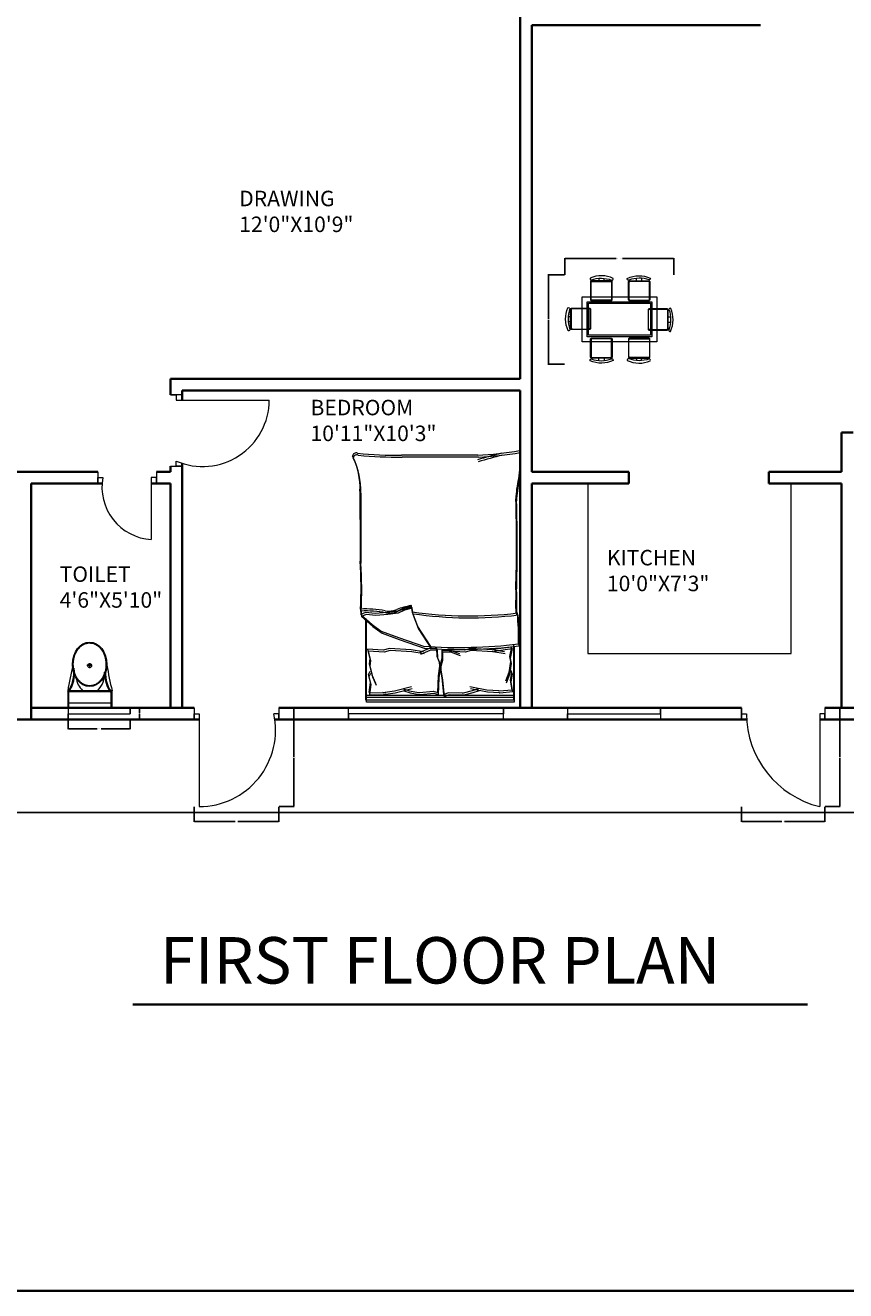
# Model space of a CAD drawing. Units: inches. Extents: x 1520 to 3401, y 1570 to 3432.
# Tile 2 of 15: x 1829 to 2147, y 1570 to 2061. Entities that reach past the tile are written whole.
import ezdxf

# ---------------------------------------------------------------- set-up
doc = ezdxf.new("R2010")
doc.units = ezdxf.units.IN
for name, color, linetype, lineweight in [('A-ANNO-DIMS', 2, 'Continuous', 18), ('A-ANNO-TITL', 7, 'Continuous', 35), ('A-ANNO-TTLB', 7, 'Continuous', 35), ('A-AREA-IDEN', 7, 'Continuous', 18), ('A-DOOR', 3, 'Continuous', 18), ('A-FLOR-CASE', 8, 'Continuous', 18), ('A-FLOR-EDGE', 7, 'Continuous', 25), ('A-FLOR-FIXT', 9, 'Continuous', 18), ('A-FURN', 8, 'Continuous', 13), ('A-GLAZ', 4, 'Continuous', 18), ('A-WALL', 7, 'Continuous', 35)]:
    doc.layers.add(name, color=color, linetype=linetype, lineweight=lineweight)
doc.styles.get("Standard").update_dxf_attribs({"font": 'arial.ttf'})
doc.dimstyles.get("Standard").update_dxf_attribs({"dimtxt": 0.18, "dimasz": 0.18, "dimexe": 0.18, "dimexo": 0.0625, "dimgap": 0.09, "dimtad": 0, "dimtih": 1, "dimtoh": 1, "dimdec": 4, "dimzin": 0, "dimdsep": 46, "dimtxsty": 'Standard', "dimcen": 0.09, "dimadec": 0, "dimazin": 0, "dimtfac": 1, "dimtdec": 4, "dimtofl": 0, "dimtmove": 0, "dimatfit": 3, "dimfxl": 1, "dimtolj": 1, "dimtzin": 0, "dimarcsym": 0})

# ---------------------------------------------------------------- blocks, each defined once
blk = doc.blocks.new('A$C31115884')
for p, q in [((283, 498), (223, 498)), ((258, 466), (258, 523)), ((0, 200), (0, 0)), ((520, 200), (0, 200)), ((10, 190), (10, 10)), ((510, 190), (10, 190)), ((510, 10), (510, 190)), ((520, 0), (520, 200)), ((510, 54), (0, 54)), ((10, 10), (510, 10)), ((0, 0), (520, 0))]:
    blk.add_line(p, q)
blk.add_circle((256, 496), 23.6)
for centre, radius, start, end in [((2778, -205), 2807, 165.4549, 171.7133), ((-295, 403), 365, 324.2091, 9.3499), ((-295, 403), 375, 324.2091, 9.3499), ((806, 403), 365, 170.6501, 215.7909), ((3237, 905), 2807, 188.2867, 194.5451), ((384, 406), 293, 190.2774, 224.1564), ((139, 406), 293, 315.8436, 2.6563), ((806, 403), 375, 179.2036, 215.7909)]:
    blk.add_arc(centre, radius, start, end)
blk.add_ellipse((256, 510), major_axis=(0, -261), ratio=0.772727)
blk.add_open_spline([(256, 259), (263, 259), (270, 260), (288, 262), (299, 265), (320, 273), (330, 278), (350, 291), (360, 299), (378, 316), (386, 326), (402, 347), (409, 358), (421, 383), (427, 395), (436, 422), (440, 436), (445, 465), (447, 480), (448, 509), (448, 524), (445, 553), (443, 568), (436, 596), (432, 610), (422, 636), (416, 649), (402, 672), (395, 683), (379, 703), (370, 712), (351, 728), (341, 735), (321, 746), (310, 751), (289, 757), (278, 759), (256, 761), (245, 761), (223, 757), (212, 754), (191, 746), (181, 741), (161, 728), (151, 720), (133, 703), (125, 693), (110, 672), (103, 660), (90, 636), (85, 623), (76, 596), (72, 582), (67, 553), (66, 538), (64, 509), (65, 494), (68, 465), (70, 450), (77, 422), (81, 408), (91, 382), (97, 370), (111, 346), (118, 335), (135, 316), (144, 307), (162, 291), (172, 284), (193, 273), (203, 269), (225, 262), (236, 260), (250, 259), (253, 259), (256, 259)], degree=3, knots=[0, 0, 0, 0, 0.110105, 0.110105, 0.285049, 0.285049, 0.459994, 0.459994, 0.634938, 0.634938, 0.809882, 0.809882, 0.984827, 0.984827, 1.159771, 1.159771, 1.334715, 1.334715, 1.50966, 1.50966, 1.684604, 1.684604, 1.859549, 1.859549, 2.034493, 2.034493, 2.209437, 2.209437, 2.384382, 2.384382, 2.559326, 2.559326, 2.73427, 2.73427, 2.909215, 2.909215, 3.084159, 3.084159, 3.259103, 3.259103, 3.434048, 3.434048, 3.608992, 3.608992, 3.783936, 3.783936, 3.958881, 3.958881, 4.133825, 4.133825, 4.30877, 4.30877, 4.483714, 4.483714, 4.658658, 4.658658, 4.833603, 4.833603, 5.008547, 5.008547, 5.183491, 5.183491, 5.358436, 5.358436, 5.53338, 5.53338, 5.708324, 5.708324, 5.883269, 5.883269, 6.058213, 6.058213, 6.233158, 6.233158, 6.283185, 6.283185, 6.283185, 6.283185])
blk = doc.blocks.new('DOOR-SWING-24-12')
for p, q in [((0, 26.25), (0, 21.75)), ((22.75, 26.25), (22.75, 21.75)), ((0, 21.75), (0, 24)), ((0, 24), (2, 24)), ((22.75, 24), (20.75, 24)), ((20.75, 24), (20.75, 0)), ((22.75, 21.75), (22.75, 24))]:
    blk.add_line(p, q)
blk.add_arc((21.91, 20.23), 20.26, 169.2703, 266.7379)
blk = doc.blocks.new('DOOR-SWING-36-13')
for p, q in [((4.5, 27.75), (0, 27.75)), ((0, 27.75), (2.25, 27.75)), ((2.25, 27.75), (2.25, 25.75)), ((2.25, 25.75), (38.25, 25.75)), ((0, 0.11), (4.5, 0.11)), ((2.25, 0.11), (2.25, 2.11)), ((4.5, 0.11), (2.25, 0.11))]:
    blk.add_line(p, q)
blk.add_arc((12.49, 25.75), 25.76, 246.5862, 0)
blk = doc.blocks.new('DOOR-SWING-36-28')
for p, q in [((0, 33.75), (0, 38.25)), ((0, 38.25), (0, 33.75)), ((0, 33.75), (0, 36)), ((0, 36), (2, 36)), ((32.37, 36), (30.37, 36)), ((30.37, 36), (30.37, 0)), ((32.37, 38.25), (32.37, 33.75)), ((32.37, 33.75), (32.37, 36))]:
    blk.add_line(p, q)
blk.add_arc((39.03, 36), 37.03, 180, 256.471)
blk = doc.blocks.new('DOOR-SWING-36-29')
for p, q in [((0, 38.25), (0, 34.72)), ((0, 33.75), (0, 36)), ((0, 36), (2, 36)), ((0, 34.72), (0, 33.75)), ((2, 36), (2, 0)), ((32.89, 36), (30.89, 36)), ((32.89, 38.25), (32.89, 33.75)), ((32.89, 33.75), (32.89, 36))]:
    blk.add_line(p, q)
blk.add_arc((2, 29.59), 29.59, 270, 12.5041)
blk = doc.blocks.new('WIN-PLAN-60-02')
for p, q in [((4.5, 60), (0, 60)), ((0, 60), (2.25, 60)), ((2.25, 60), (2.25, 0)), ((4.5, 0), (0, 0)), ((2.25, 0), (4.5, 0))]:
    blk.add_line(p, q)
blk = doc.blocks.new('WIN-PLAN-36-04')
for p, q in [((0, 4.5), (0, 0)), ((0, 0), (0, 2.25)), ((0, 2.25), (36, 2.25)), ((36, 2.25), (36, 4.5)), ((36, 4.5), (36, 0))]:
    blk.add_line(p, q)
blk = doc.blocks.new('WIN-PLAN-24-06')
for p, q in [((0, 4.5), (0, 0)), ((0, 0), (0, 2.25)), ((0, 2.25), (24, 2.25)), ((24, 2.25), (24, 4.5)), ((24, 4.5), (24, 2.25))]:
    blk.add_line(p, q)
blk = doc.blocks.new('KITCHEN-COUNTER-02')
for p, q in [((0, 65.95), (0, 0)), ((78.77, 0), (78.77, 65.95)), ((0, 0), (78.77, 0))]:
    blk.add_line(p, q)
blk = doc.blocks.new('DINING-SET-6-SEAT')
for points in [[(9.94, 32.23, -0.175809), (17.84, 32.17, 0.578392), (18.44, 32.83, 0.214524), (9.52, 32.95, 0.552014), (9.94, 32.23, -0.065079)], [(17.51, 31.92), (10.17, 31.92, 0.414214), (9.66, 31.4), (9.66, 24.66, 0.414214), (10.17, 24.14), (17.51, 24.14, 0.414214), (18.02, 24.66), (18.02, 31.4, 0.414214), (17.51, 31.92)], [(14.93, 31.92), (14.93, 32.84, -0.064759)], [(24.5, 32.17, -0.578392), (23.9, 32.83, -0.214524), (32.82, 32.95, -0.552014), (32.4, 32.23, 0.175809), (24.5, 32.17)], [(32.17, 31.92, -0.414214), (32.68, 31.4), (32.68, 24.66, -0.414214), (32.17, 24.14), (24.83, 24.14, -0.414214), (24.32, 24.66), (24.32, 31.4, -0.414214), (24.83, 31.92), (32.17, 31.92)], [(27.41, 31.92), (27.41, 32.84, 0.064759)], [(1.67, 13.15, -0.578392), (1.02, 12.55, -0.214524), (0.9, 21.47, -0.552014), (1.61, 21.05, 0.175809), (1.67, 13.15)], [(1.93, 20.82, -0.414214), (2.45, 21.33), (9.19, 21.33, -0.414214), (9.7, 20.82), (9.7, 13.49, -0.414214), (9.19, 12.97), (2.45, 12.97, -0.414214), (1.93, 13.49), (1.93, 20.82)], [(39.71, 20.57, 0.414214), (39.19, 21.08), (32.45, 21.08, 0.414214), (31.94, 20.57), (31.94, 13.23, 0.414214), (32.45, 12.72), (39.19, 12.72, 0.414214), (39.71, 13.23), (39.71, 20.57)], [(40.02, 20.8, -0.175809), (39.96, 12.9, 0.578392), (40.62, 12.3, 0.214524), (40.74, 21.22, 0.552014), (40.02, 20.8, -0.065079)], [(1.93, 16.06), (1, 16.06, 0.064759)], [(39.71, 15.81), (40.63, 15.81, -0.064759)], [(17.51, 1.93), (10.17, 1.93, -0.414214), (9.66, 2.45), (9.66, 9.19, -0.414214), (10.17, 9.7), (17.51, 9.7, -0.414214), (18.02, 9.19), (18.02, 2.45, -0.414214), (17.51, 1.93)], [(32.17, 1.93, 0.414214), (32.68, 2.45), (32.68, 9.19, 0.414214), (32.17, 9.7), (24.83, 9.7, 0.414214), (24.32, 9.19), (24.32, 2.45, 0.414214), (24.83, 1.93), (32.17, 1.93)], [(17.84, 1.67, -0.578392), (18.44, 1.02, -0.214524), (9.52, 0.9, -0.552014), (9.94, 1.61, 0.175809), (17.84, 1.67)], [(14.93, 1.93), (14.93, 1, 0.064759)], [(32.4, 1.61, -0.175809), (24.5, 1.67, 0.578392), (23.9, 1.02, 0.214524), (32.82, 0.9, 0.552014), (32.4, 1.61, -0.065079)], [(27.41, 1.93), (27.41, 1, -0.064759)]]:
    blk.add_lwpolyline(points, format="xyb")
for points in [[(10.18, 31.68), (17.28, 31.68, -0.414214), (17.79, 31.17), (17.79, 24.89, -0.414214), (17.28, 24.37), (10.18, 24.37, -0.512069), (9.89, 24.89), (9.89, 31.17, -0.512069)], [(32.16, 31.68), (25.06, 31.68, 0.414214), (24.55, 31.17), (24.55, 24.89, 0.414214), (25.06, 24.37), (32.16, 24.37, 0.512069), (32.45, 24.89), (32.45, 31.17, 0.512069)], [(2.16, 20.82), (2.16, 13.72, 0.414214), (2.68, 13.2), (8.96, 13.2, 0.414214), (9.47, 13.72), (9.47, 20.82, 0.512069), (8.96, 21.1), (2.68, 21.1, 0.512069)], [(39.48, 20.57), (39.48, 13.47, -0.414214), (38.96, 12.95), (32.68, 12.95, -0.414214), (32.17, 13.47), (32.17, 20.57, -0.512069), (32.68, 20.85), (38.96, 20.85, -0.512069)], [(10.18, 2.16), (17.28, 2.16, 0.414214), (17.79, 2.68), (17.79, 8.96, 0.414214), (17.28, 9.47), (10.18, 9.47, 0.512069), (9.89, 8.96), (9.89, 2.68, 0.512069)], [(32.16, 2.16), (25.06, 2.16, -0.414214), (24.55, 2.68), (24.55, 8.96, -0.414214), (25.06, 9.47), (32.16, 9.47, -0.512069), (32.45, 8.96), (32.45, 2.68, -0.512069)]]:
    blk.add_lwpolyline(points, format="xyb", close=True)
for points in [[(12.88, 32.86), (12.88, 31.92)], [(29.46, 32.86), (29.46, 31.92)], [(0.99, 18.12), (1.93, 18.12)], [(40.65, 17.86), (39.71, 17.86)], [(12.88, 0.99), (12.88, 1.93)], [(29.46, 0.99), (29.46, 1.93)]]:
    blk.add_lwpolyline(points)
for points in [[(6.35, 25.72), (35.36, 25.72), (35.36, 8.31), (6.35, 8.31)], [(8.29, 23.79), (33.43, 23.79), (33.43, 10.25), (8.29, 10.25)], [(8.87, 23.21), (32.85, 23.21), (32.85, 10.83), (8.87, 10.83)]]:
    blk.add_lwpolyline(points, close=True)
blk = doc.blocks.new('*D135')
at = {"layer": 'A-ANNO-DIMS', "color": 0, "lineweight": -2, "transparency": 16777216}
for p, q in [((2139.24, 1796.18), (2145.09, 1796.18)), ((2144.91, 1796), (2144.91, 1777.24)), ((2144.91, 1758.11), (2144.91, 1776.87)), ((2139.24, 1757.93), (2145.09, 1757.93))]:
    blk.add_line(p, q, dxfattribs=at)
at = {"layer": 'A-ANNO-DIMS', "color": 0, "transparency": 16777216}
for points in [[(2144.88, 1796), (2144.94, 1796), (2144.91, 1796.18)], [(2144.88, 1758.11), (2144.94, 1758.11), (2144.91, 1757.93)]]:
    blk.add_solid(points, dxfattribs=at)
at = {"layer": 'Defpoints', "color": 0, "transparency": 16777216}
for p in [(2139.17, 1796.18), (2144.91, 1796.18), (2139.17, 1757.93)]:
    blk.add_point(p, dxfattribs=at)
at = {"layer": 'A-ANNO-DIMS', "color": 0, "transparency": 16777216, "insert": (2144.91, 1777.05), "char_height": 0.18, "attachment_point": 5}
blk.add_mtext('\\A1;D28 38 TYP.', dxfattribs=at)
blk = doc.blocks.new('*D136')
at = {"layer": 'A-ANNO-DIMS', "color": 0, "lineweight": -2, "transparency": 16777216}
for p, q in [((2106.81, 1757.87), (2106.81, 1752.01)), ((2139.17, 1757.87), (2139.17, 1752.01)), ((2106.99, 1752.19), (2122.46, 1752.19)), ((2138.99, 1752.19), (2123.52, 1752.19))]:
    blk.add_line(p, q, dxfattribs=at)
at = {"layer": 'A-ANNO-DIMS', "color": 0, "transparency": 16777216}
for points in [[(2106.99, 1752.22), (2106.99, 1752.16), (2106.81, 1752.19)], [(2138.99, 1752.22), (2138.99, 1752.16), (2139.17, 1752.19)]]:
    blk.add_solid(points, dxfattribs=at)
at = {"layer": 'Defpoints', "color": 0, "transparency": 16777216}
for p in [(2106.81, 1757.93), (2139.17, 1757.93), (2139.17, 1752.19)]:
    blk.add_point(p, dxfattribs=at)
at = {"layer": 'A-ANNO-DIMS', "color": 0, "transparency": 16777216, "insert": (2122.99, 1752.19), "char_height": 0.18, "attachment_point": 5}
blk.add_mtext('\\A1;32 TYP.', dxfattribs=at)
blk = doc.blocks.new('*D137')
at = {"layer": 'A-ANNO-DIMS', "color": 0, "lineweight": -2, "transparency": 16777216}
for p, q in [((1927.68, 1796.18), (1933.53, 1796.18)), ((1933.35, 1796), (1933.35, 1777.24)), ((1933.35, 1758.11), (1933.35, 1776.87)), ((1927.68, 1757.93), (1933.53, 1757.93))]:
    blk.add_line(p, q, dxfattribs=at)
at = {"layer": 'A-ANNO-DIMS', "color": 0, "transparency": 16777216}
for points in [[(1933.32, 1796), (1933.38, 1796), (1933.35, 1796.18)], [(1933.32, 1758.11), (1933.38, 1758.11), (1933.35, 1757.93)]]:
    blk.add_solid(points, dxfattribs=at)
at = {"layer": 'Defpoints', "color": 0, "transparency": 16777216}
for p in [(1927.62, 1796.18), (1933.35, 1796.18), (1927.62, 1757.93)]:
    blk.add_point(p, dxfattribs=at)
at = {"layer": 'A-ANNO-DIMS', "color": 0, "transparency": 16777216, "insert": (1933.35, 1777.05), "char_height": 0.18, "attachment_point": 5}
blk.add_mtext('\\A1;D29 38 TYP.', dxfattribs=at)
blk = doc.blocks.new('*D138')
at = {"layer": 'A-ANNO-DIMS', "color": 0, "lineweight": -2, "transparency": 16777216}
for p, q in [((1894.73, 1757.87), (1894.73, 1752.01)), ((1927.62, 1757.87), (1927.62, 1752.01)), ((1894.91, 1752.19), (1910.64, 1752.19)), ((1927.44, 1752.19), (1911.7, 1752.19))]:
    blk.add_line(p, q, dxfattribs=at)
at = {"layer": 'A-ANNO-DIMS', "color": 0, "transparency": 16777216}
for points in [[(1894.91, 1752.22), (1894.91, 1752.16), (1894.73, 1752.19)], [(1927.44, 1752.22), (1927.44, 1752.16), (1927.62, 1752.19)]]:
    blk.add_solid(points, dxfattribs=at)
at = {"layer": 'Defpoints', "color": 0, "transparency": 16777216}
for p in [(1894.73, 1757.93), (1927.62, 1757.93), (1927.62, 1752.19)]:
    blk.add_point(p, dxfattribs=at)
at = {"layer": 'A-ANNO-DIMS', "color": 0, "transparency": 16777216, "insert": (1911.17, 1752.19), "char_height": 0.18, "attachment_point": 5}
blk.add_mtext('\\A1;33 TYP.', dxfattribs=at)
blk = doc.blocks.new('*D143')
at = {"layer": 'A-ANNO-DIMS', "color": 0, "lineweight": -2, "transparency": 16777216}
for p, q in [((1845.96, 1791.62), (1845.96, 1787.9)), ((1869.96, 1791.62), (1869.96, 1787.9)), ((1846.14, 1788.08), (1857.2, 1788.08)), ((1869.78, 1788.08), (1858.71, 1788.08))]:
    blk.add_line(p, q, dxfattribs=at)
at = {"layer": 'A-ANNO-DIMS', "color": 0, "transparency": 16777216}
for points in [[(1846.14, 1788.11), (1846.14, 1788.05), (1845.96, 1788.08)], [(1869.78, 1788.11), (1869.78, 1788.05), (1869.96, 1788.08)]]:
    blk.add_solid(points, dxfattribs=at)
at = {"layer": 'Defpoints', "color": 0, "transparency": 16777216}
for p in [(1845.96, 1791.68), (1869.96, 1791.68), (1869.96, 1788.08)]:
    blk.add_point(p, dxfattribs=at)
at = {"layer": 'A-ANNO-DIMS', "color": 0, "transparency": 16777216, "insert": (1857.96, 1788.08), "char_height": 0.18, "attachment_point": 5}
blk.add_mtext('\\A1;W6 24 TYP.', dxfattribs=at)
blk = doc.blocks.new('*D144')
at = {"layer": 'A-ANNO-DIMS', "color": 0, "lineweight": -2, "transparency": 16777216}
for p, q in [((1870.02, 1796.18), (1873.74, 1796.18)), ((1873.56, 1796), (1873.56, 1794.11)), ((1870.02, 1791.68), (1873.74, 1791.68)), ((1873.56, 1791.86), (1873.56, 1793.75))]:
    blk.add_line(p, q, dxfattribs=at)
at = {"layer": 'A-ANNO-DIMS', "color": 0, "transparency": 16777216}
for points in [[(1873.53, 1796), (1873.59, 1796), (1873.56, 1796.18)], [(1873.53, 1791.86), (1873.59, 1791.86), (1873.56, 1791.68)]]:
    blk.add_solid(points, dxfattribs=at)
at = {"layer": 'Defpoints', "color": 0, "transparency": 16777216}
for p in [(1869.96, 1796.18), (1873.56, 1796.18), (1869.96, 1791.68)]:
    blk.add_point(p, dxfattribs=at)
at = {"layer": 'A-ANNO-DIMS', "color": 0, "transparency": 16777216, "insert": (1873.56, 1793.93), "char_height": 0.18, "attachment_point": 5}
blk.add_mtext('\\A1;5 TYP.', dxfattribs=at)
blk = doc.blocks.new('*D173')
at = {"layer": 'A-ANNO-DIMS', "color": 0, "lineweight": -2, "transparency": 16777216}
for p, q in [((2038.36, 1964.02), (2038.36, 1970.49)), ((2038.54, 1970.31), (2058.24, 1970.31)), ((2080.5, 1970.31), (2060.8, 1970.31)), ((2080.68, 1964.02), (2080.68, 1970.49))]:
    blk.add_line(p, q, dxfattribs=at)
at = {"layer": 'A-ANNO-DIMS', "color": 0, "transparency": 16777216}
for points in [[(2038.54, 1970.34), (2038.54, 1970.28), (2038.36, 1970.31)], [(2080.5, 1970.34), (2080.5, 1970.28), (2080.68, 1970.31)]]:
    blk.add_solid(points, dxfattribs=at)
at = {"layer": 'Defpoints', "color": 0, "transparency": 16777216}
for p in [(2080.68, 1970.31), (2038.36, 1963.96), (2080.68, 1963.96)]:
    blk.add_point(p, dxfattribs=at)
at = {"layer": 'A-ANNO-DIMS', "color": 0, "transparency": 16777216, "insert": (2059.52, 1970.31), "char_height": 0.18, "attachment_point": 5}
blk.add_mtext('\\A1;DINING SET 42 TYP.', dxfattribs=at)
blk = doc.blocks.new('*D174')
at = {"layer": 'A-ANNO-DIMS', "color": 0, "lineweight": -2, "transparency": 16777216}
for p, q in [((2038.3, 1963.96), (2031.83, 1963.96)), ((2032.01, 1963.78), (2032.01, 1946.88)), ((2032.01, 1929.61), (2032.01, 1946.52)), ((2038.3, 1929.43), (2031.83, 1929.43))]:
    blk.add_line(p, q, dxfattribs=at)
at = {"layer": 'A-ANNO-DIMS', "color": 0, "transparency": 16777216}
for points in [[(2031.98, 1963.78), (2032.04, 1963.78), (2032.01, 1963.96)], [(2031.98, 1929.61), (2032.04, 1929.61), (2032.01, 1929.43)]]:
    blk.add_solid(points, dxfattribs=at)
at = {"layer": 'Defpoints', "color": 0, "transparency": 16777216}
for p in [(2032.01, 1963.96), (2038.36, 1963.96), (2038.36, 1929.43)]:
    blk.add_point(p, dxfattribs=at)
at = {"layer": 'A-ANNO-DIMS', "color": 0, "transparency": 16777216, "insert": (2032.01, 1946.7), "char_height": 0.18, "attachment_point": 5}
blk.add_mtext('\\A1;35 TYP.', dxfattribs=at)

msp = doc.modelspace()

# ---------------------------------------------------------------- linework, layer by layer
at = {"layer": 'A-ANNO-TITL'}
msp.add_line((1871.0735, 1681.3063), (2132.3813, 1681.3063), dxfattribs=at)
at = {"layer": 'A-ANNO-TTLB'}
msp.add_lwpolyline([(1519.9253, 3431.7421), (3400.8761, 3431.7421), (3400.8761, 1570.3458), (1519.9253, 1570.3458)], close=True, dxfattribs=at)
at = {"layer": 'A-FLOR-EDGE'}
msp.add_line((1699.6128, 1755.6786), (2339.6128, 1755.6786), dxfattribs=at)
at = {"layer": 'A-FURN'}
for p, q in [((2004.6418, 1894.1124), (1975.1333, 1894.1124)), ((2004.9156, 1893.346), (1975.4071, 1893.346)), ((1959.2246, 1834.464), (1959.3198, 1832.3724, 4.6408)), ((1976.0163, 1834.7846), (1973.6026, 1833.6712)), ((1976.2901, 1834.0181), (1973.8764, 1832.9048)), ((1978.9871, 1835.5268), (1976.0163, 1834.7846)), ((1979.2609, 1834.7604), (1976.2901, 1834.0181)), ((1979.3585, 1833.1146), (1978.9871, 1835.5268)), ((1979.6322, 1832.3481), (1979.2609, 1834.7604)), ((1961.1627, 1833.1146), (1959.3198, 1832.3724)), ((1959.3198, 1832.3724), (1963.7621, 1828.4757)), ((1959.4984, 1833.6975), (1959.5936, 1831.6059, 4.6408)), ((1961.4365, 1832.3481), (1959.5936, 1831.6059)), ((1959.5936, 1831.6059), (1964.0358, 1827.7093)), ((1964.8761, 1832.7435), (1961.1627, 1833.1146)), ((1961.2407, 1799.1089), (1961.2407, 1831.0105)), ((1965.1499, 1831.9771), (1961.4365, 1832.3481)), ((1961.5145, 1798.3425), (1961.5145, 1830.244)), ((1969.5179, 1833.1146), (1964.8761, 1832.7435)), ((1969.7917, 1832.3481), (1965.1499, 1831.9771)), ((1973.6026, 1833.6712), (1969.5179, 1833.1146)), ((1973.8764, 1832.9048), (1969.7917, 1832.3481)), ((1981.4008, 1827.7335), (1979.3585, 1833.1146)), ((1981.6746, 1826.9671), (1979.6322, 1832.3481)), ((1963.7621, 1828.4757), (1967.2898, 1825.878)), ((1964.0358, 1827.7093), (1967.5636, 1825.1115)), ((1967.2898, 1825.878), (1973.974, 1823.4657)), ((1967.5636, 1825.1115), (1974.2478, 1822.6993)), ((1986.4241, 1819.9491), (1981.4008, 1827.7335)), ((1986.6979, 1819.1827), (1981.6746, 1826.9671)), ((1970.4231, 1819.1614), (1968.0729, 1818.4935)), ((1978.827, 1818.6446), (1970.4231, 1819.1614)), ((1973.974, 1823.4657), (1983.9702, 1819.9491)), ((1974.2478, 1822.6993), (1984.244, 1819.1827)), ((1985.8354, 1819.1773), (1982.1544, 1817.6368)), ((1988.7758, 1819.361), (1985.8354, 1819.1773)), ((1988.9763, 1816.1527), (1988.7758, 1819.361)), ((2001.8122, 1819.1614), (1999.462, 1818.4935)), ((2010.2161, 1818.6446), (2001.8122, 1819.1614)), ((2011.5747, 1819.0318), (2017.6848, 1819.8985)), ((2017.6848, 1819.8985), (2016.9916, 1816.085)), ((2018.5344, 1820.8207), (2018.5344, 1799.1089)), ((2018.8082, 1820.0543), (2018.8082, 1798.3425)), ((1968.0729, 1818.4935), (1961.9206, 1818.9774)), ((1961.9206, 1818.9774), (1962.8503, 1815.2145)), ((1968.3467, 1817.727), (1962.1944, 1818.2109)), ((1962.1944, 1818.2109), (1963.1241, 1814.4481)), ((1962.8503, 1815.2145), (1962.6233, 1813.2899)), ((1963.1241, 1814.4481), (1962.8971, 1812.5235)), ((1970.6968, 1818.395), (1968.3467, 1817.727)), ((1979.1008, 1817.8781), (1970.6968, 1818.395)), ((1983.6607, 1817.8454), (1978.827, 1818.6446)), ((1983.9345, 1817.079), (1979.1008, 1817.8781)), ((1986.1092, 1818.4108), (1982.4282, 1816.8704)), ((1989.0496, 1818.5946), (1986.1092, 1818.4108)), ((1989.8087, 1813.9469), (1988.9763, 1816.1527)), ((1989.2501, 1815.3863), (1989.0496, 1818.5946)), ((1990.0825, 1813.1805), (1989.2501, 1815.3863)), ((1990.1648, 1813.1382), (1990.858, 1815.3916)), ((1990.4386, 1812.3718), (1991.1318, 1814.6252)), ((1990.858, 1815.3916), (1990.858, 1818.6062)), ((1990.858, 1818.6062), (1993.8041, 1818.6062)), ((1991.1318, 1814.6252), (1991.1318, 1817.8398)), ((1991.1318, 1817.8398), (1994.0779, 1817.8398)), ((1999.462, 1818.4935), (1993.3097, 1818.9774)), ((1999.7358, 1817.727), (1993.5835, 1818.2109)), ((1993.8041, 1818.6062), (1997.5741, 1817.2984)), ((1994.0779, 1817.8398), (1997.8478, 1816.5319)), ((2002.086, 1818.395), (1999.7358, 1817.727)), ((2010.4899, 1817.8781), (2002.086, 1818.395)), ((2010.2161, 1818.6446), (2011.5747, 1819.0318)), ((2015.0499, 1817.8454), (2010.2161, 1818.6446)), ((2010.4899, 1817.8781), (2011.8485, 1818.2653)), ((2015.3236, 1817.079), (2010.4899, 1817.8781)), ((2011.8485, 1818.2653), (2017.9586, 1819.132)), ((2016.9916, 1816.085), (2017.3382, 1814.1783)), ((2017.9586, 1819.132), (2017.2654, 1815.3186)), ((2017.2654, 1815.3186), (2017.612, 1813.4118)), ((1962.3639, 1809.1054), (1962.9801, 1810.3597)), ((1962.6233, 1813.2899), (1963.5855, 1809.0081)), ((1962.6377, 1808.339), (1963.2539, 1809.5932)), ((1962.8971, 1812.5235), (1963.8593, 1808.2416)), ((1989.4521, 1808.5406), (1989.906, 1812.3899)), ((1989.7259, 1807.7742), (1990.1798, 1811.6235)), ((1989.906, 1812.3899), (1989.8087, 1813.9469)), ((1990.1798, 1811.6235), (1990.0825, 1813.1805)), ((1990.1648, 1811.5782), (1990.1648, 1813.1382)), ((1990.858, 1807.7647), (1990.1648, 1811.5782)), ((1990.4386, 1810.8117), (1990.4386, 1812.3718)), ((1991.1318, 1806.9982), (1990.4386, 1810.8117)), ((2016.645, 1809.8448), (2015.4319, 1806.5513)), ((2017.3382, 1814.1783), (2016.645, 1809.8448)), ((2017.612, 1813.4118), (2016.9188, 1809.0783)), ((2017.8581, 1810.0181), (2017.1649, 1811.2315)), ((2017.3382, 1806.898), (2017.8581, 1810.0181)), ((2018.1319, 1809.2517), (2017.4387, 1810.465)), ((1963.0774, 1806.0238), (1962.3639, 1809.1054)), ((1962.6235, 1802.1745), (1963.0774, 1806.0238)), ((1963.3512, 1805.2574), (1962.6377, 1808.339)), ((1962.8973, 1801.4081), (1963.3512, 1805.2574)), ((1963.5855, 1809.0081), (1965.0017, 1805.7967)), ((1963.8593, 1808.2416), (1965.2755, 1805.0303)), ((1989.1603, 1802.0963), (1989.4521, 1808.5406)), ((1989.4341, 1801.3298), (1989.7259, 1807.7742)), ((1991.5512, 1801.3511), (1990.858, 1807.7647)), ((1991.825, 1800.5847), (1991.1318, 1806.9982)), ((2016.9188, 1809.0783), (2015.7057, 1805.7849)), ((2018.0314, 1803.0845), (2017.3382, 1806.898)), ((2017.612, 1806.1315), (2018.1319, 1809.2517)), ((2018.3052, 1802.3181), (2017.612, 1806.1315)), ((2018.5344, 1800.9475), (1961.2407, 1800.9475)), ((2018.8082, 1800.1811), (1961.5145, 1800.1811)), ((1962.6235, 1802.1745), (1969.1001, 1802.0583)), ((1962.8973, 1801.4081), (1969.3739, 1801.2918)), ((1967.898, 1802.1568), (1972.4513, 1802.7887)), ((1969.1001, 1802.0583), (1967.898, 1802.1568)), ((1968.1718, 1801.3904), (1972.7251, 1802.0223)), ((1969.3739, 1801.2918), (1968.1718, 1801.3904)), ((1972.4513, 1802.7887), (1978.9482, 1804.4105)), ((1972.7251, 1802.0223), (1979.222, 1803.6441)), ((1975.7052, 1803.5131), (1978.1807, 1802.7995)), ((1975.9789, 1802.7467), (1978.4545, 1802.033)), ((1978.1807, 1802.7995), (1981.6941, 1802.1507)), ((1978.4545, 1802.033), (1981.9679, 1801.3842)), ((1981.6941, 1802.1507), (1982.0789, 1802.1747)), ((1981.9679, 1801.3842), (1982.3527, 1801.4083)), ((1982.0789, 1802.1747), (1987.3874, 1802.6802)), ((1982.3527, 1801.4083), (1987.6612, 1801.9137)), ((1987.3874, 1802.6802), (1989.1603, 1802.0963)), ((1987.6612, 1801.9137), (1989.4341, 1801.3298)), ((1993.2842, 1802.0445), (1991.5512, 1801.3511)), ((1993.558, 1801.278), (1991.825, 1800.5847)), ((1998.6139, 1801.8711), (1993.2842, 1802.0445)), ((1998.8877, 1801.1047), (1993.558, 1801.278)), ((1998.9995, 1801.8711), (1998.6139, 1801.8711)), ((1999.2733, 1801.1047), (1998.8877, 1801.1047)), ((2002.4655, 1802.7378), (1998.9995, 1801.8711)), ((2002.7393, 1801.9714), (1999.2733, 1801.1047)), ((2008.1845, 1803.0845), (2001.599, 1804.2979)), ((2008.4583, 1802.3181), (2001.8728, 1803.5314)), ((2004.8917, 1803.6045), (2002.4655, 1802.7378)), ((2005.1655, 1802.8381), (2002.7393, 1801.9714)), ((2012.7683, 1802.7378), (2008.1845, 1803.0845)), ((2013.0421, 1801.9714), (2008.4583, 1802.3181)), ((2012.8946, 1802.716), (2012.7683, 1802.7378)), ((2018.0267, 1803.1108), (2012.8946, 1802.716)), ((2013.1684, 1801.9495), (2013.0421, 1801.9714)), ((2018.3004, 1802.3443), (2013.1684, 1801.9495)), ((2018.5344, 1799.1089), (1961.2407, 1799.1089)), ((2018.8082, 1798.3425), (1961.5145, 1798.3425))]:
    msp.add_line(p, q, dxfattribs=at)
for centre, radius, start, end in [((1957.4709, 1893.663), 1.3216, 62.658759, 176.020019), ((1931.3989, 1881.4303), 27.6519, 357.471365, 26.468093), ((1957.7447, 1892.8965), 1.3216, 62.658759, 176.020019), ((1931.6727, 1880.6638), 27.6519, 357.471365, 26.468093), ((1973.3654, 2053.5985), 159.4958, 264.499804, 270.635087), ((1973.6392, 2052.832), 159.4958, 264.499804, 270.635087), ((2043.347, 1770.6818), 127.6292, 103.38322, 107.705328), ((1997.013, 2039.8841), 145.9712, 272.995782, 279.409071), ((2043.6208, 1769.9154), 127.6292, 103.38322, 107.705328), ((1997.2868, 2039.1177), 145.9712, 272.995782, 279.409071), ((2021.3968, 1894.6793), 1.3056, 102.562578, 113.478142), ((2048.6673, 1883.3595), 28.2474, 167.282939, 176.652001), ((2054.9494, 1876.4534), 35.5269, 166.064841, 178.911252), ((2055.2232, 1875.687), 35.5269, 166.064841, 178.911252), ((2048.9411, 1882.5931), 28.2474, 170.117434, 176.652001), ((7428.0425, 1880.4172), 5469.0186, 180.0021678, 180.2868875), ((7428.3163, 1879.6508), 5469.0186, 180.0021678, 180.2868875), ((1441.4676, 1859.7878), 578.2214, 358.2277093, 1.7185413), ((1441.7414, 1859.0214), 578.2214, 358.2277093, 1.7185413), ((1804.1898, 1842.6456), 155.2505, 356.979123, 3.836453), ((1804.4636, 1841.8792), 155.2505, 356.979123, 3.836453), ((2223.2784, 1836.4818), 203.9381, 178.476202, 181.008194), ((2223.5522, 1835.7153), 203.9381, 178.476202, 181.008194), ((1961.1665, 1791.1292), 43.3783, 79.876284, 92.565707), ((1970.2584, 1841.1485), 7.4621, 258.660801, 293.738416), ((1985.3517, 1800.8859), 35.5505, 100.66171, 109.880578), ((1985.6255, 1800.1195), 35.5505, 100.66171, 109.880578), ((1978.7789, 1835.6016), 0.2212, 340.246365, 91.137655), ((1979.0527, 1834.8351), 0.2212, 340.246365, 91.137655), ((1961.4402, 1790.3627), 43.3783, 79.876284, 92.565707), ((1970.5322, 1840.3821), 7.4621, 258.660801, 293.738416), ((2001.414, 1986.51), 154.6762, 261.784488, 276.900621), ((2001.6878, 1985.7435), 154.6762, 261.784488, 276.900621), ((1920.6038, 1823.2016), 99.8715, 358.721776, 5.603971), ((1920.8776, 1822.4352), 99.8715, 358.721776, 5.603971), ((1997.0944, 2017.3641), 197.7742, 266.086548, 276.78213), ((1997.3682, 2016.5976), 197.7742, 266.086548, 276.78213)]:
    msp.add_arc(centre, radius, start, end, dxfattribs=at)
at = {"layer": 'A-WALL'}
for p, q in [((2021.1128, 1923.6786), (2021.1128, 2234.1786)), ((2025.6128, 2060.6786), (2114.2382, 2060.6786)), ((2025.6128, 2060.6786), (2025.6128, 1887.6786)), ((2114.2382, 2060.6786), (2025.6128, 2060.6786)), ((2021.1128, 1923.6786), (2021.1128, 2052.6786)), ((1885.6128, 1919.1786), (1885.6128, 1923.6786)), ((1885.6128, 1923.6786), (2021.1128, 1923.6786)), ((1885.6128, 1917.4716), (1885.6128, 1919.1786)), ((2021.1128, 1919.1786), (1890.1128, 1919.1786)), ((1890.1128, 1919.1786), (1890.1128, 1915.4716)), ((2021.1128, 1796.1786), (2021.1128, 1919.1786)), ((2150.1128, 1902.917), (2145.6128, 1902.917)), ((2145.6128, 1902.917), (2145.6128, 1887.6786)), ((1885.6128, 1887.6786), (1885.6128, 1889.8302)), ((1890.1128, 1890.9783), (1890.1128, 1887.6786)), ((1857.4148, 1887.6786), (1796.9488, 1887.6786)), ((1831.6128, 1883.1786), (1831.6128, 1791.6786)), ((1859.1178, 1883.1786), (1831.6128, 1883.1786)), ((1885.6128, 1883.1786), (1878.1684, 1883.1786)), ((1885.6128, 1887.6786), (1880.1684, 1887.6786)), ((1885.6128, 1796.1786), (1885.6128, 1883.1786)), ((1890.1128, 1887.6786), (1890.1128, 1796.1786)), ((2063.2346, 1887.6786), (2025.6128, 1887.6786)), ((2025.6128, 1883.1786), (2063.2346, 1883.1786)), ((2025.6128, 1883.1786), (2025.6128, 1796.1786)), ((2063.2346, 1883.1786), (2025.6128, 1883.1786)), ((2063.2346, 1887.6786), (2063.2346, 1883.1786)), ((2145.6128, 1887.6786), (2117.4929, 1887.6786)), ((2117.4929, 1887.6786), (2117.4929, 1883.1786)), ((2145.6128, 1883.1786), (2117.4929, 1883.1786)), ((2117.4929, 1883.1786), (2145.6128, 1883.1786)), ((2145.6128, 1883.1786), (2145.6128, 1796.1786)), ((1831.6128, 1796.1786), (1885.6128, 1796.1786)), ((1894.7277, 1796.1786), (1831.6128, 1796.1786)), ((1890.1128, 1796.1786), (1894.7277, 1796.1786)), ((2106.8084, 1796.1786), (1927.6174, 1796.1786)), ((1927.6174, 1796.1786), (2021.1128, 1796.1786)), ((2213.4538, 1796.1786), (2139.1737, 1796.1786)), ((2145.6128, 1796.1786), (2150.1128, 1796.1786)), ((1896.7277, 1791.6786), (1704.1128, 1791.6786)), ((2108.8768, 1791.6786), (1926.0259, 1791.6786)), ((2215.4538, 1791.6786), (2137.1737, 1791.6786))]:
    msp.add_line(p, q, dxfattribs=at)

# ---------------------------------------------------------------- block references
at = {"layer": 'A-DOOR'}
for name, p in [('DOOR-SWING-36-13', (1885.613, 1889.717)), ('DOOR-SWING-24-12', (1857.415, 1861.429)), ('DOOR-SWING-36-29', (1894.728, 1757.93)), ('DOOR-SWING-36-28', (2106.808, 1757.929))]:
    msp.add_blockref(name, p, dxfattribs=at)
at = {"layer": 'A-FLOR-CASE'}
msp.add_blockref('KITCHEN-COUNTER-02', (2047.269, 1817.227), dxfattribs=at)
at = {"layer": 'A-FLOR-FIXT', "xscale": 0.0330640103915726, "yscale": 0.0330640103915726, "zscale": 0.0330640103915726}
msp.add_blockref('A$C31115884', (1845.8162, 1796.1786), dxfattribs=at)
at = {"layer": 'A-FURN'}
msp.add_blockref('DINING-SET-6-SEAT', (2038.702, 1929.774), dxfattribs=at)
at = {"layer": 'A-GLAZ'}
for name, p in [('WIN-PLAN-24-06', (1845.955, 1791.679)), ('WIN-PLAN-36-04', (2039.494, 1791.679))]:
    msp.add_blockref(name, p, dxfattribs=at)
at = {"layer": 'A-GLAZ', "rotation": 270}
msp.add_blockref('WIN-PLAN-60-02', (1954.6423, 1796.1785), dxfattribs=at)

# ---------------------------------------------------------------- texts
at = {"layer": 'A-ANNO-TITL', "insert": (1881.505, 1707.3539), "char_height": 18, "attachment_point": 1}
msp.add_mtext_dynamic_manual_height_columns('FIRST FLOOR PLAN ', width=486.836858, gutter_width=12.5, heights=[0], dxfattribs=at)
at = {"layer": 'A-AREA-IDEN', "char_height": 6, "attachment_point": 1}
for s, width, insert in [('DRAWING\\P12\'0"X10\'9"', 68.680212, (1912.2357, 1996.5696)), ('BEDROOM\\P10\'11"X10\'3"', 190.565236, (1939.8575, 1915.5627)), ('KITCHEN\\P10\'0"X7\'3"', 88.358055, (2054.7025, 1857.4026)), ('TOILET\\P4\'6"X5\'10"', 102.758842, (1842.6856, 1851.0036))]:
    msp.add_mtext_dynamic_manual_height_columns(s, width=width, gutter_width=12.5, heights=[0], dxfattribs=dict(at, insert=insert))

# ---------------------------------------------------------------- dimensions: what is measured, and where the dimension line sits
at = {"layer": 'A-ANNO-DIMS'}
for base, p1, p2, text, picture, middle in [((2080.6819, 1970.31), (2038.3611, 1963.9619), (2080.6819, 1963.9619), 'DINING SET <> TYP.', '*D173', (2059.5215, 1970.31)), ((1869.9552, 1788.0786), (1845.9552, 1791.6786), (1869.9552, 1791.6786), 'W6 <> TYP.', '*D143', (1857.9552, 1788.0786)), ((1927.6174, 1752.193), (1894.7277, 1757.9303), (1927.6174, 1757.9303), '<> TYP.', '*D138', (1911.1726, 1752.193)), ((2139.1737, 1752.1911), (2106.8084, 1757.9286), (2139.1737, 1757.9286), '<> TYP.', '*D136', (2122.991, 1752.1911))]:
    dim = msp.add_linear_dim(base=base, p1=p1, p2=p2, text=text, dimstyle='Standard', override={"dimdec": 0, "dimlfac": 1, "dimrnd": 0, "dimzin": 0, "dimdsep": 46, "dimlunit": 2}, dxfattribs=at)
    dim.commit()
    dim.dimension.update_dxf_attribs({"geometry": picture, "text_midpoint": middle})
for base, p1, p2, text, picture, middle in [((2032.013, 1963.9619), (2038.3611, 1929.4331), (2038.3611, 1963.9619), '<> TYP.', '*D174', (2032.013, 1946.6975)), ((1873.5552017428, 1796.1786294992), (1869.9552017428, 1791.6786294992), (1869.9552017428, 1796.1786294992), '<> TYP.', '*D144', (1873.5552017428, 1793.9286294992)), ((1933.3546, 1796.1786), (1927.6174, 1757.9303), (1927.6174, 1796.1786), 'D29 <> TYP.', '*D137', (1933.3546, 1777.0545)), ((2144.9112, 1796.1786), (2139.1737, 1757.9286), (2139.1737, 1796.1786), 'D28 <> TYP.', '*D135', (2144.9112, 1777.0536))]:
    dim = msp.add_linear_dim(base=base, p1=p1, p2=p2, angle=90, text=text, dimstyle='Standard', override={"dimdec": 0, "dimlfac": 1, "dimrnd": 0, "dimzin": 0, "dimdsep": 46, "dimlunit": 2}, dxfattribs=at)
    dim.commit()
    dim.dimension.update_dxf_attribs({"geometry": picture, "text_midpoint": middle})

doc.saveas('drawing.dxf')
